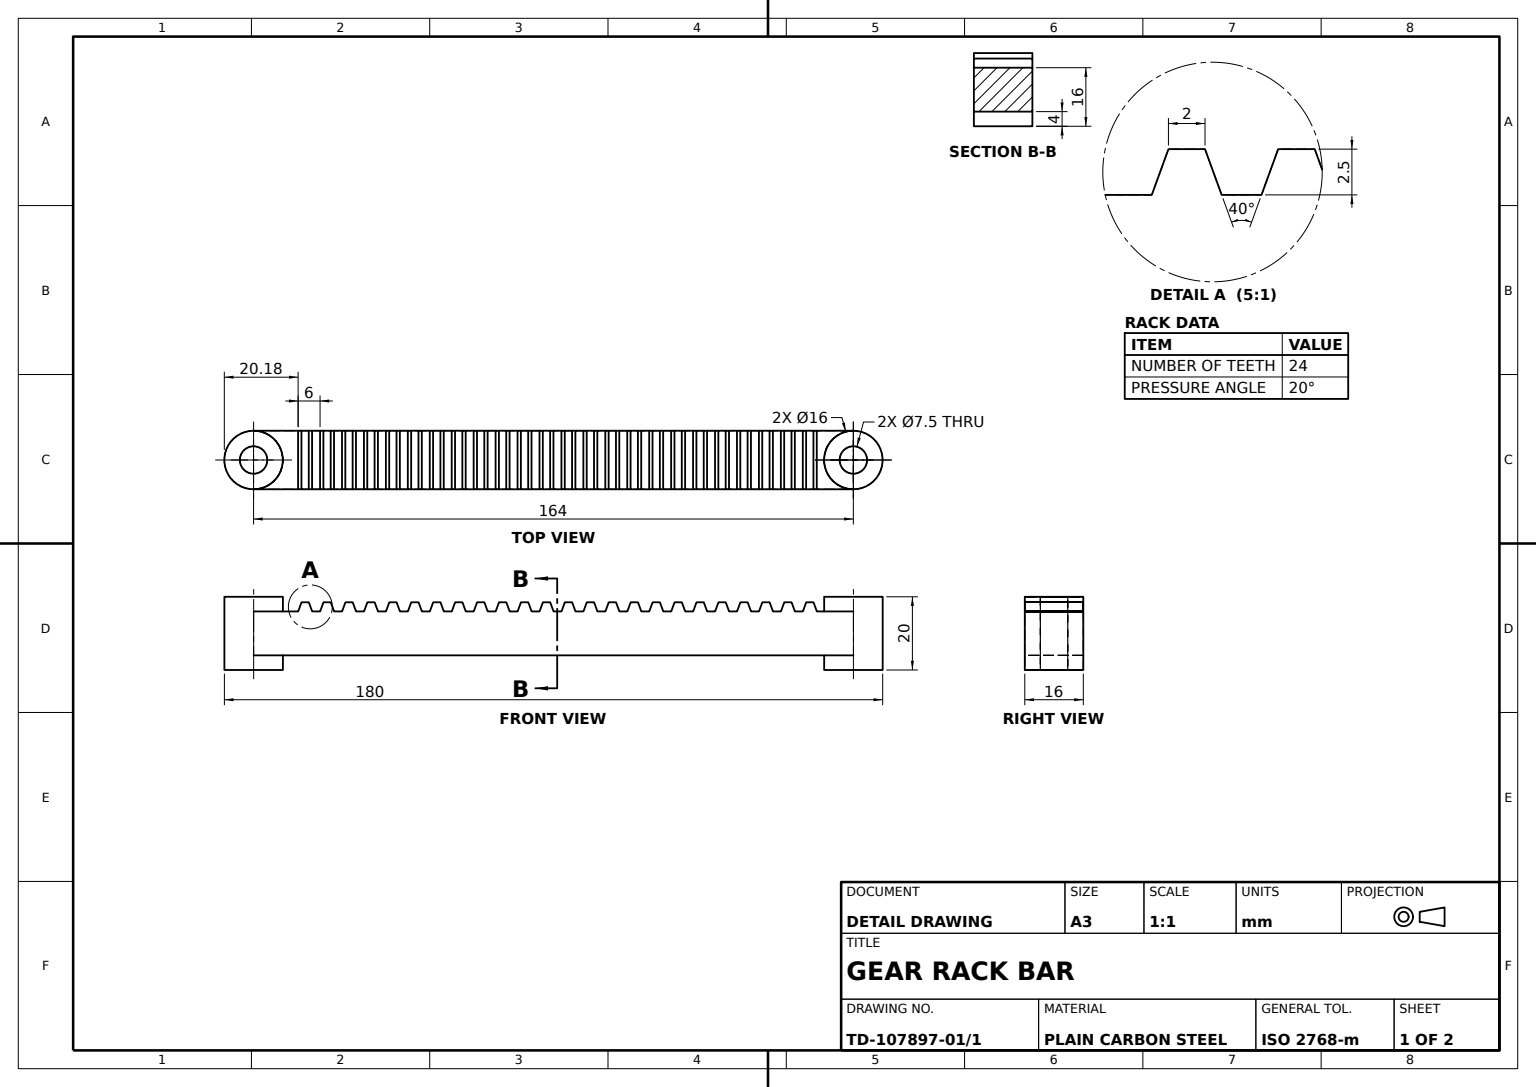
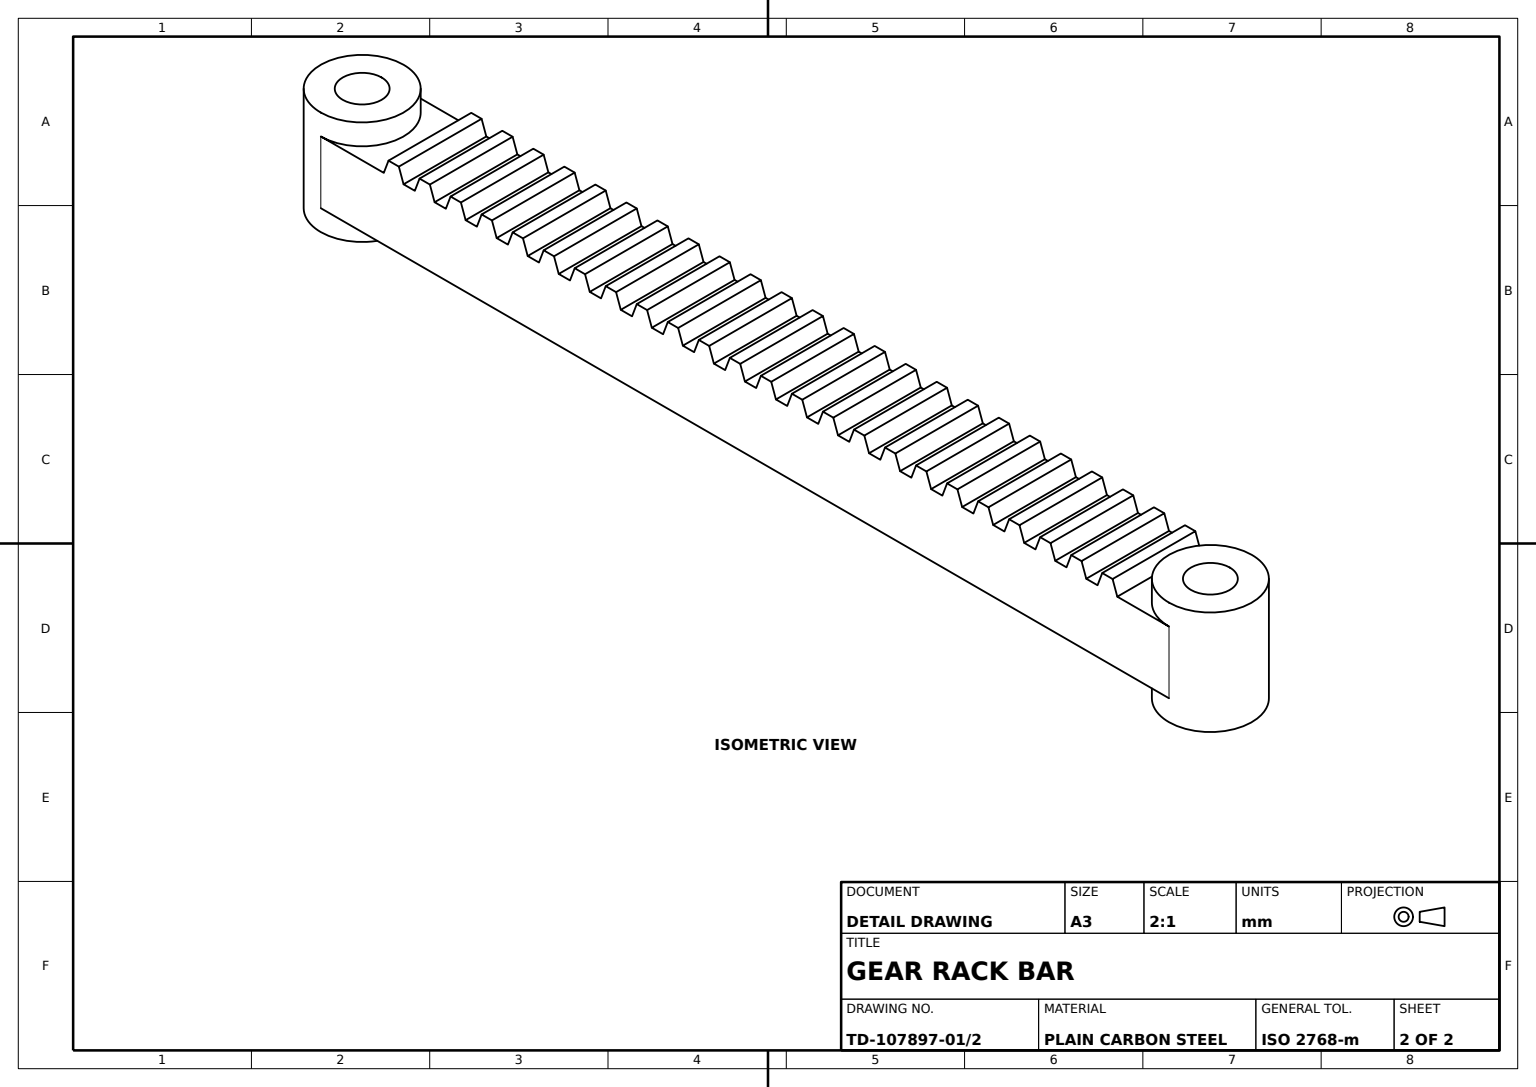
SolidWorks part; units mm, degrees
material "Plain Carbon Steel"
ref_plane "Front Plane" through (0, 0, 0) normal (0, 0, 1) x (1, 0, 0)
ref_plane "Top Plane" through (0, 0, 0) normal (0, 1, 0) x (1, 0, 0)
ref_plane "Right Plane" through (0, 0, 0) normal (1, 0, 0) x (0, 0, -1)
sketch "End Bosses Sketch" plane through (0, 0, 0) normal (0, 1, 0) x (1, 0, 0)
  line L0 (-82, 0) -> (82, 0) construction
  circle A0 centre (-82, 0) radius 3.75
  circle A1 centre (82, 0) radius 3.75
  circle A2 centre (-82, 0) radius 8
  circle A3 centre (82, 0) radius 8
  point P4 (0, 0)
  dimension "D1" = 16
  dimension "D2" = 7.5
  dimension "D3" = 16
  dimension "D4" = 7.5
  dimension "D5" = 164
extrude "End Bosses" add sketch "End Bosses Sketch" along normal blind 20
ref_plane "Plane1" through (0, 0, 0) normal (0, 0, 1) x (1, 0, 0)
sketch "Rack Tooth Profile Sketch" plane through (0, 0, 0) normal (0, 0, 1) x (1, 0, 0)
  line L0 (-82, 0) -> (-82, 36.9629) construction
  line L1 (-90, 0) -> (-74, 0) construction
  line L2 (82, 0) -> (82, 27.2635) construction
  line L3 (74, 0) -> (90, 0) construction
  line L4 (-74, 20) -> (-90, 20) construction
  line L5 (-82, 4) -> (82, 4)
  line L6 (-82, 4) -> (-82, 16)
  line L7 (-82, 16) -> (-69.8199, 16)
  line L8 (82, 4) -> (82, 16)
  line L9 (72, 16) -> (71.0901, 18.5)
  line L10 (71.0901, 18.5) -> (69.0901, 18.5)
  line L11 (69.0901, 18.5) -> (68.1801, 16)
  line L12 (90, 0) -> (90, 20) construction
  line L13 (65.0901, 18.5) -> (63.0901, 18.5)
  line L14 (66, 16) -> (65.0901, 18.5)
  line L15 (63.0901, 18.5) -> (62.1801, 16)
  line L16 (60, 16) -> (62.1801, 16)
  line L17 (66, 16) -> (68.1801, 16)
  line L18 (66, 16) -> (65.0901, 18.5)
  line L19 (65.0901, 18.5) -> (63.0901, 18.5)
  line L20 (63.0901, 18.5) -> (62.1801, 16)
  line L21 (60, 16) -> (59.0901, 18.5)
  line L22 (59.0901, 18.5) -> (57.0901, 18.5)
  line L23 (57.0901, 18.5) -> (56.1801, 16)
  line L24 (54, 16) -> (53.0901, 18.5)
  line L25 (53.0901, 18.5) -> (51.0901, 18.5)
  line L26 (51.0901, 18.5) -> (50.1801, 16)
  line L27 (48, 16) -> (47.0901, 18.5)
  line L28 (47.0901, 18.5) -> (45.0901, 18.5)
  line L29 (45.0901, 18.5) -> (44.1801, 16)
  line L30 (42, 16) -> (41.0901, 18.5)
  line L31 (41.0901, 18.5) -> (39.0901, 18.5)
  line L32 (39.0901, 18.5) -> (38.1801, 16)
  line L33 (36, 16) -> (35.0901, 18.5)
  line L34 (35.0901, 18.5) -> (33.0901, 18.5)
  line L35 (33.0901, 18.5) -> (32.1801, 16)
  line L36 (30, 16) -> (29.0901, 18.5)
  line L37 (29.0901, 18.5) -> (27.0901, 18.5)
  line L38 (27.0901, 18.5) -> (26.1801, 16)
  line L39 (24, 16) -> (23.0901, 18.5)
  line L40 (23.0901, 18.5) -> (21.0901, 18.5)
  line L41 (21.0901, 18.5) -> (20.1801, 16)
  line L42 (18, 16) -> (17.0901, 18.5)
  line L43 (17.0901, 18.5) -> (15.0901, 18.5)
  line L44 (15.0901, 18.5) -> (14.1801, 16)
  line L45 (12, 16) -> (11.0901, 18.5)
  line L46 (11.0901, 18.5) -> (9.0901, 18.5)
  line L47 (9.0901, 18.5) -> (8.1801, 16)
  line L48 (6, 16) -> (5.0901, 18.5)
  line L49 (5.0901, 18.5) -> (3.0901, 18.5)
  line L50 (3.0901, 18.5) -> (2.1801, 16)
  line L51 (0, 16) -> (-0.9099, 18.5)
  line L52 (-0.9099, 18.5) -> (-2.9099, 18.5)
  line L53 (-2.9099, 18.5) -> (-3.8199, 16)
  line L54 (-6, 16) -> (-6.9099, 18.5)
  line L55 (-6.9099, 18.5) -> (-8.9099, 18.5)
  line L56 (-8.9099, 18.5) -> (-9.8199, 16)
  line L57 (-12, 16) -> (-12.9099, 18.5)
  line L58 (-12.9099, 18.5) -> (-14.9099, 18.5)
  line L59 (-14.9099, 18.5) -> (-15.8199, 16)
  line L60 (-18, 16) -> (-18.9099, 18.5)
  line L61 (-18.9099, 18.5) -> (-20.9099, 18.5)
  line L62 (-20.9099, 18.5) -> (-21.8199, 16)
  line L63 (-24, 16) -> (-24.9099, 18.5)
  line L64 (-24.9099, 18.5) -> (-26.9099, 18.5)
  line L65 (-26.9099, 18.5) -> (-27.8199, 16)
  line L66 (-30, 16) -> (-30.9099, 18.5)
  line L67 (-30.9099, 18.5) -> (-32.9099, 18.5)
  line L68 (-32.9099, 18.5) -> (-33.8199, 16)
  line L69 (-36, 16) -> (-36.9099, 18.5)
  line L70 (-36.9099, 18.5) -> (-38.9099, 18.5)
  line L71 (-38.9099, 18.5) -> (-39.8199, 16)
  line L72 (-42, 16) -> (-42.9099, 18.5)
  line L73 (-42.9099, 18.5) -> (-44.9099, 18.5)
  line L74 (-44.9099, 18.5) -> (-45.8199, 16)
  line L75 (-48, 16) -> (-48.9099, 18.5)
  line L76 (-48.9099, 18.5) -> (-50.9099, 18.5)
  line L77 (-50.9099, 18.5) -> (-51.8199, 16)
  line L78 (-54, 16) -> (-54.9099, 18.5)
  line L79 (-54.9099, 18.5) -> (-56.9099, 18.5)
  line L80 (-56.9099, 18.5) -> (-57.8199, 16)
  line L81 (-60, 16) -> (-60.9099, 18.5)
  line L82 (-60.9099, 18.5) -> (-62.9099, 18.5)
  line L83 (-62.9099, 18.5) -> (-63.8199, 16)
  line L84 (-66, 16) -> (-66.9099, 18.5)
  line L85 (-66.9099, 18.5) -> (-68.9099, 18.5)
  line L86 (-68.9099, 18.5) -> (-69.8199, 16)
  line L87 (72, 16) -> (82, 16)
  line L88 (54, 16) -> (56.1801, 16)
  line L89 (48, 16) -> (50.1801, 16)
  line L90 (42, 16) -> (44.1801, 16)
  line L91 (36, 16) -> (38.1801, 16)
  line L92 (30, 16) -> (32.1801, 16)
  line L93 (24, 16) -> (26.1801, 16)
  line L94 (18, 16) -> (20.1801, 16)
  line L95 (12, 16) -> (14.1801, 16)
  line L96 (6, 16) -> (8.1801, 16)
  line L97 (0, 16) -> (2.1801, 16)
  line L98 (-6, 16) -> (-3.8199, 16)
  line L99 (-12, 16) -> (-9.8199, 16)
  line L100 (-18, 16) -> (-15.8199, 16)
  line L101 (-24, 16) -> (-21.8199, 16)
  line L102 (-30, 16) -> (-27.8199, 16)
  line L103 (-36, 16) -> (-33.8199, 16)
  line L104 (-42, 16) -> (-39.8199, 16)
  line L105 (-48, 16) -> (-45.8199, 16)
  line L106 (-54, 16) -> (-51.8199, 16)
  line L107 (-60, 16) -> (-57.8199, 16)
  line L108 (-66, 16) -> (-63.8199, 16)
  dimension "D1" = 4
  dimension "D2" = 4
  dimension "D3" = 18
  dimension "D4" = 2
  dimension "D5" = 2.5
  dimension "D6" = 2.5
  dimension "D7" = 2
  dimension "D8" = 40
  dimension "D10" = 6
  dimension "D12" = 40
  dimension "D13" = 24
extrude "Rack Teeth 24x" add sketch "Rack Tooth Profile Sketch" along normal mid plane 16 contours L108 L84 L85 L86 L7 L6 L5 L8 L87 L9 L10 L11 L17 L14 L13 L15 L16 L21 L22 L23 L88 L24 L25 L26 L89 L27 L28 L29 L90 L30 L31 L32 L91 L33 L34 L35 L92 L36 L37 L38 L93 L39 L40 L41 L94 L42 L43 L44 L95 L45 L46
sketch "Pin Holes Sketch" plane through (0, 20, 0) normal (0, 1, 0) x (1, 0, 0)
  circle A0 centre (-82, 0) radius 3.75
  circle A1 centre (82, 0) radius 3.75
  dimension "D1" = 7.5
extrude "Pin Holes 2x" cut sketch "Pin Holes Sketch" against normal blind 36
